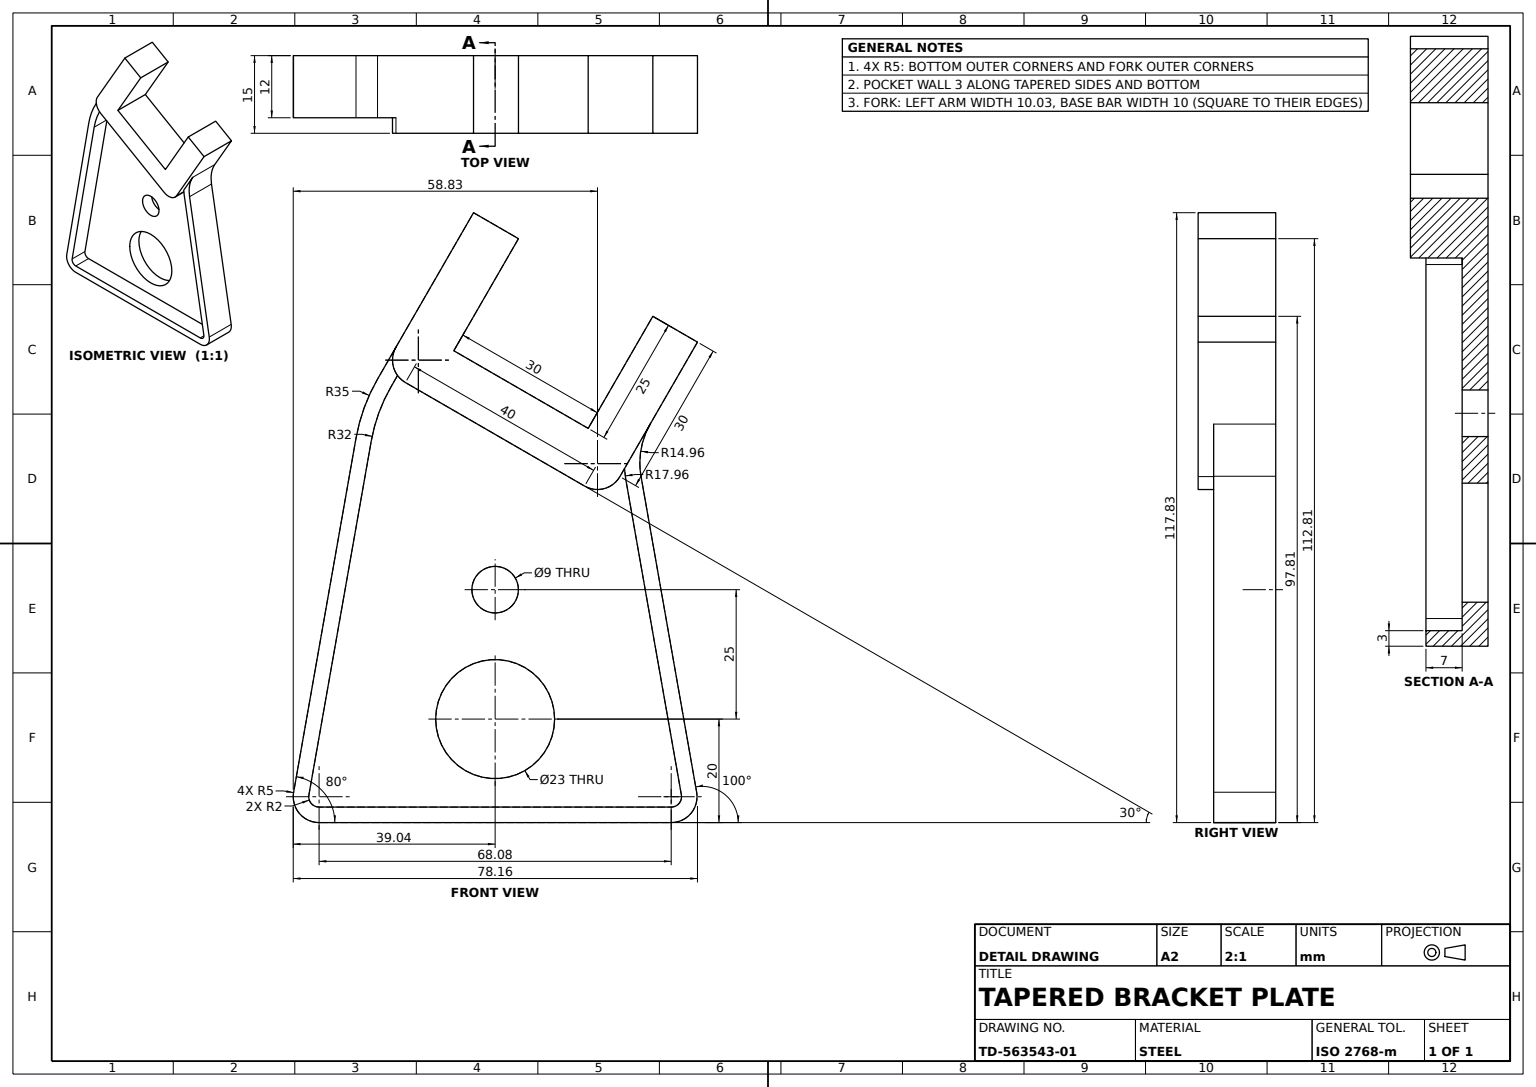
from build123d import *

# Parameters (mm, degrees)
FORK_BOSS_15MM_DEPTH           = 15
SKETCH1_10_R                   = 11.5
SKETCH1_10_R_2                 = 4.5
PLATE_BOSS_12MM_DEPTH          = 12
POCKET_START                   = -7
POCKET_AND_HOLES_CUT_7MM_DEPTH = 7


with BuildPart() as part:
    # Bracket Outline Sketch → Fork Boss 15mm (new body)
    with BuildSketch(Plane.XY):
        with BuildLine():
            Line((-17.348851567, 85.016364122), (17.292164585, 65.016364122))
            ThreePointArc((17.292164585, 65.016364122), (21.08625981, 64.51686201), (24.122291604, 66.846491141))
            Line((24.122291604, 66.846491141), (29.979005279, 76.990616791))
            Line((29.979005279, 76.990616791), (39.122291604, 92.827253255))
            Line((39.122291604, 92.827253255), (30.490381057, 97.810889132))
            Line((30.490381057, 97.810889132), (17.990381057, 76.160254038))
            Line((17.990381057, 76.160254038), (-7.990381057, 91.160254038))
            Line((-7.990381057, 91.160254038), (4.509618943, 112.810889132))
            Line((4.509618943, 112.810889132), (-4.178978585, 117.827253255))
            Line((-4.178978585, 117.827253255), (-19.178978585, 91.846491141))
            ThreePointArc((-19.178978585, 91.846491141), (-19.678480698, 88.052395915), (-17.348851567, 85.016364122))
        make_face()
    extrude(amount=FORK_BOSS_15MM_DEPTH)

    # Sketch1_10 → Plate Boss 12mm (add)
    with BuildSketch(Plane.XY):
        with BuildLine():
            ThreePointArc((24.122291604, 66.846491141), (21.08625981, 64.51686201), (17.292164585, 65.016364122))
            Line((17.292164585, 65.016364122), (-17.348851567, 85.016364122))
            ThreePointArc((-17.348851567, 85.016364122), (-19.678480698, 88.052395915), (-19.178978585, 91.846491141))
            Line((-19.178978585, 91.846491141), (-22.741186866, 85.676565412))
            ThreePointArc((-22.741186866, 85.676565412), (-25.323096431, 80.149782404), (-26.906195607, 74.258654802))
            Line((-26.906195607, 74.258654802), (-38.965270802, 5.868240888))
            ThreePointArc((-38.965270802, 5.868240888), (-37.871454253, 1.786061952), (-34.041232037, 0))
            Line((-34.041232037, 0), (34.041232037, 0))
            ThreePointArc((34.041232037, 0), (37.871454253, 1.786061952), (38.965270802, 5.868240888))
            Line((38.965270802, 5.868240888), (28.201741138, 66.911250985))
            ThreePointArc((28.201741138, 66.911250985), (28.201741138, 72.107623698), (29.979005279, 76.990616791))
            Line((29.979005279, 76.990616791), (24.122291604, 66.846491141))
        make_face()
        with Locations((0, 20)):
            Circle(SKETCH1_10_R, mode=Mode.SUBTRACT)
        with Locations((0, 45)):
            Circle(SKETCH1_10_R_2, mode=Mode.SUBTRACT)
    extrude(amount=PLATE_BOSS_12MM_DEPTH)

    # Pocket and Holes Sketch → Pocket and Holes Cut 7mm (cut)
    with BuildSketch(Plane.XY.offset(12).offset(POCKET_START)):
        with BuildLine():
            Line((25.009745942, 68.383607145), (24.122291604, 66.846491141))
            ThreePointArc((24.122291604, 66.846491141), (21.08625981, 64.51686201), (17.292164585, 65.016364122))
            Line((17.292164585, 65.016364122), (-17.348851567, 85.016364122))
            ThreePointArc((-17.348851567, 85.016364122), (-18.180803852, 85.618476392), (-18.872189895, 86.377863731))
            Line((-18.872189895, 86.377863731), (-20.143109976, 84.176565019))
            ThreePointArc((-20.143109976, 84.176565019), (-22.504396013, 79.122684974), (-23.952156408, 73.735536834))
            Line((-23.952156408, 73.735536834), (-36.010847543, 5.347296355))
            ThreePointArc((-36.010847543, 5.347296355), (-35.573320923, 3.714424781), (-34.041232037, 3))
            Line((-34.041232037, 3), (34.041232037, 3))
            ThreePointArc((34.041232037, 3), (35.573320923, 3.714424781), (36.010847543, 5.347296355))
            Line((36.010847543, 5.347296355), (25.247317879, 66.390306452))
            ThreePointArc((25.247317879, 66.390306452), (25.100664631, 67.383635431), (25.009745942, 68.383607145))
        make_face()
    extrude(amount=POCKET_AND_HOLES_CUT_7MM_DEPTH, mode=Mode.SUBTRACT)


solid = part.part
